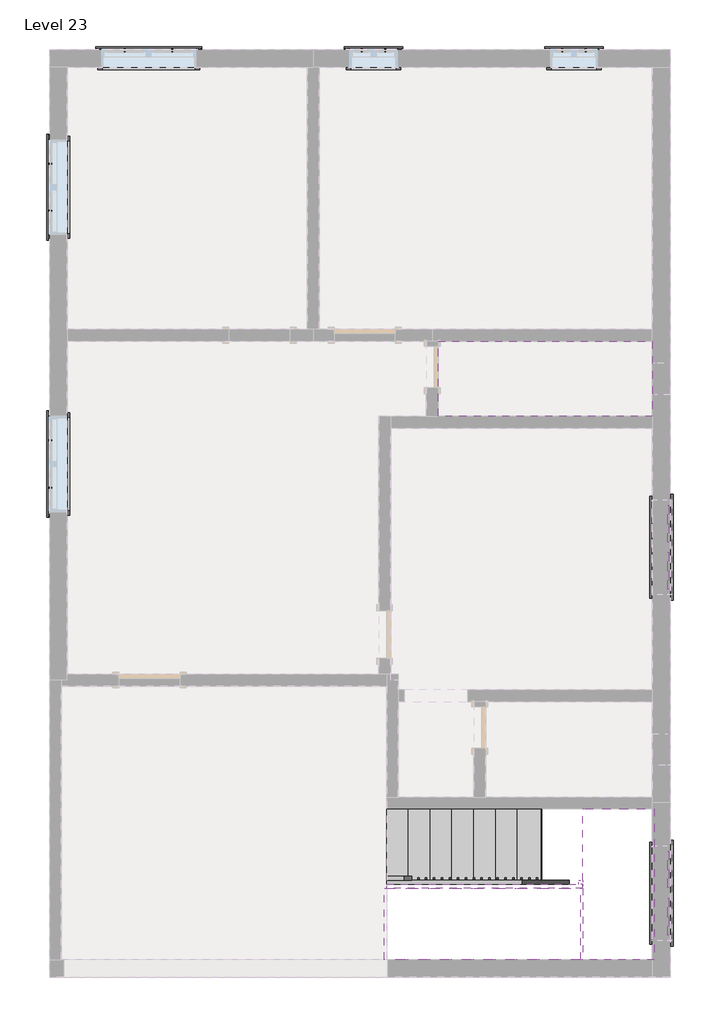
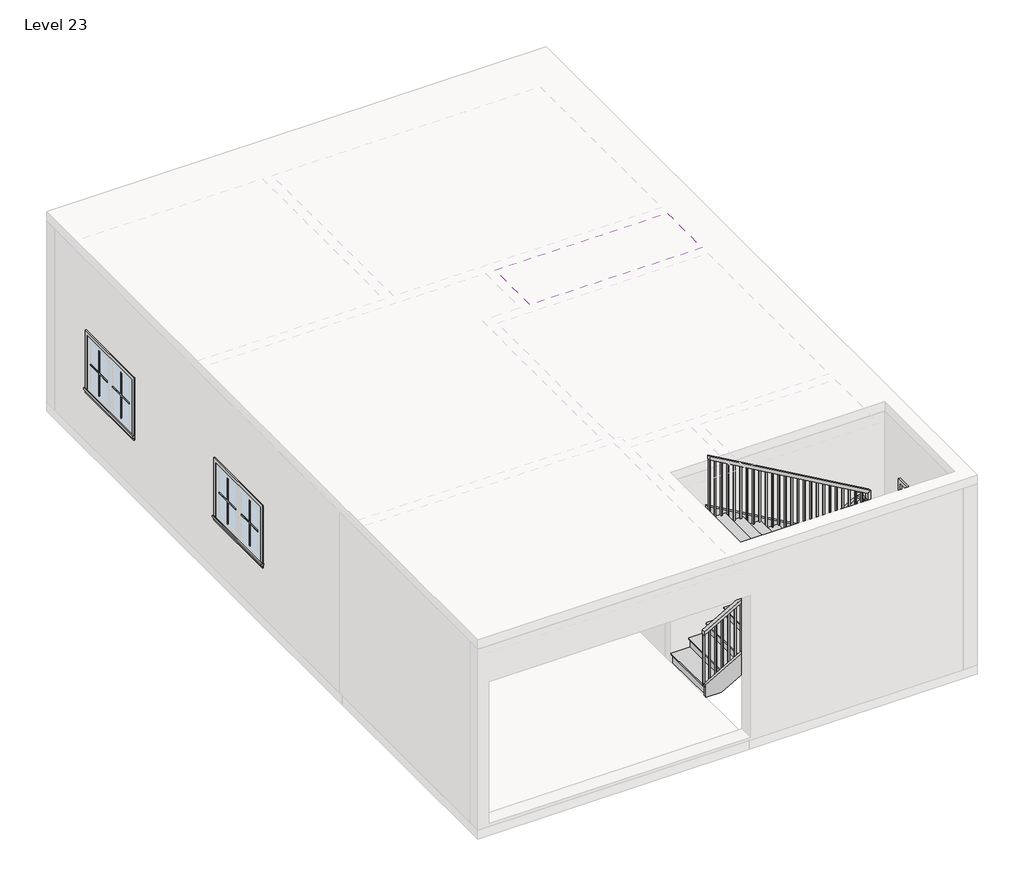
# One storey, part 2 of 2: 44 proxies, 3 members, 2 stair flights, 1 covering, 1 railing, 1 slab.
"""IFC4 building model written with IfcOpenShell, lengths in millimetres."""

from ifc_helpers import new_model, si_unit, frame, origin, place, context, project, spatial, polyline, outline, extrude, faceted_brep, transform, mapped, element, save
from components import muntin_pattern_2x2_muntin_pattern_2x2_2357e71d, muntin_pattern_2x2_muntin_pattern_2x2_302d8f29, muntin_pattern_2x2_muntin_pattern_2x2_53152e2c, muntin_pattern_2x2_muntin_pattern_2x2_e8f3e573, trim_window_exterior_flat_with_sill_c4e67c73, trim_window_exterior_flat_with_sill_a665a915, trim_window_interior_flat_picture_frame_cf1733af, trim_window_interior_flat_picture_frame_d485c387, non_monolithic_landing_f056e2ed, stair_flight_e0f3031c, stair_flight_f2ac7941

model = new_model("IFC4")

# Units and contexts
model_context = context("Model", 3, world=origin())
ifc_project = project(units=[si_unit("LENGTHUNIT", "METRE", prefix="MILLI")], contexts=[model_context])

# Site, building, storey
site = spatial("IfcSite", under=ifc_project)
building = spatial("IfcBuilding", under=site)
storey = spatial("IfcBuildingStorey", under=building, Name="Level 23", Elevation=19202.4)

# Proxies
placement = place(None, origin())
muntin_pattern_2x2_muntin_pattern_2x2_shape = muntin_pattern_2x2_muntin_pattern_2x2_2357e71d(model_context)
element("IfcBuildingElementProxy", 1, Name="Muntin Pattern_2x2 : Muntin Pattern_2x2", ObjectType="Muntin Pattern_2x2 : Muntin Pattern_2x2", at=placement, inside=storey, context=model_context, shape_type="MappedRepresentation", body=[
    mapped(muntin_pattern_2x2_muntin_pattern_2x2_shape, transform((-4942.3279463, 5897.3080275, 20186.65), x_axis=(1.0, 0.0, 0.0), y_axis=(0.0, 1.0, 0.0), z_axis=(0.0, 0.0, 1.0))),
])
element("IfcBuildingElementProxy", 2, Name="Muntin Pattern_2x2 : Muntin Pattern_2x2", ObjectType="Muntin Pattern_2x2 : Muntin Pattern_2x2", at=placement, inside=storey, context=model_context, shape_type="MappedRepresentation", body=[
    mapped(muntin_pattern_2x2_muntin_pattern_2x2_shape, transform((-5899.5904463, 3838.3205275, 20186.65), x_axis=(0.0, 1.0, 0.0), y_axis=(-1.0, 0.0, 0.0), z_axis=(0.0, 0.0, 1.0))),
])
element("IfcBuildingElementProxy", 3, Name="Muntin Pattern_2x2 : Muntin Pattern_2x2", ObjectType="Muntin Pattern_2x2 : Muntin Pattern_2x2", at=placement, inside=storey, context=model_context, shape_type="MappedRepresentation", body=[
    mapped(muntin_pattern_2x2_muntin_pattern_2x2_shape, transform((-5899.5904463, 293.4330275, 20186.65), x_axis=(0.0, 1.0, 0.0), y_axis=(-1.0, 0.0, 0.0), z_axis=(0.0, 0.0, 1.0))),
])
element("IfcBuildingElementProxy", 4, Name="Muntin Pattern_2x2 : Muntin Pattern_2x2", ObjectType="Muntin Pattern_2x2 : Muntin Pattern_2x2", at=placement, inside=storey, context=model_context, shape_type="MappedRepresentation", body=[
    mapped(muntin_pattern_2x2_muntin_pattern_2x2_shape, transform((2031.5595537, -166.9419725, 20491.45), x_axis=(0.0, -1.0, 0.0), y_axis=(1.0, 0.0, 0.0), z_axis=(0.0, 0.0, 1.0))),
])
element("IfcBuildingElementProxy", 5, Name="Muntin Pattern_2x2 : Muntin Pattern_2x2", ObjectType="Muntin Pattern_2x2 : Muntin Pattern_2x2", at=placement, inside=storey, context=model_context, shape_type="MappedRepresentation", body=[
    mapped(muntin_pattern_2x2_muntin_pattern_2x2_shape, transform((2031.5595537, -4599.2419725, 20491.45), x_axis=(0.0, -1.0, 0.0), y_axis=(1.0, 0.0, 0.0), z_axis=(0.0, 0.0, 1.0))),
])
element("IfcBuildingElementProxy", 6, Name="Muntin Pattern_2x2 : Muntin Pattern_2x2", ObjectType="Muntin Pattern_2x2 : Muntin Pattern_2x2", at=placement, inside=storey, context=model_context, shape_type="MappedRepresentation", body=[
    mapped(muntin_pattern_2x2_muntin_pattern_2x2_shape, transform((-4942.3279463, 5897.3080275, 20186.65), x_axis=(1.0, 0.0, 0.0), y_axis=(0.0, 1.0, 0.0), z_axis=(0.0, 0.0, 1.0))),
])
element("IfcBuildingElementProxy", 7, Name="Muntin Pattern_2x2 : Muntin Pattern_2x2", ObjectType="Muntin Pattern_2x2 : Muntin Pattern_2x2", at=placement, inside=storey, context=model_context, shape_type="MappedRepresentation", body=[
    mapped(muntin_pattern_2x2_muntin_pattern_2x2_shape, transform((2031.5595537, -4599.2419725, 20491.45), x_axis=(0.0, -1.0, 0.0), y_axis=(1.0, 0.0, 0.0), z_axis=(0.0, 0.0, 1.0))),
])
muntin_pattern_2x2_muntin_pattern_2x2_2_shape = muntin_pattern_2x2_muntin_pattern_2x2_302d8f29(model_context)
element("IfcBuildingElementProxy", 8, Name="Muntin Pattern_2x2 : Muntin Pattern_2x2", ObjectType="Muntin Pattern_2x2 : Muntin Pattern_2x2", at=placement, inside=storey, context=model_context, shape_type="MappedRepresentation", body=[
    mapped(muntin_pattern_2x2_muntin_pattern_2x2_2_shape, transform((-4335.9029463, 5897.3080275, 20186.65), x_axis=(-1.0, 0.0, 0.0), y_axis=(0.0, -1.0, 0.0), z_axis=(0.0, 0.0, 1.0))),
])
element("IfcBuildingElementProxy", 9, Name="Muntin Pattern_2x2 : Muntin Pattern_2x2", ObjectType="Muntin Pattern_2x2 : Muntin Pattern_2x2", at=placement, inside=storey, context=model_context, shape_type="MappedRepresentation", body=[
    mapped(muntin_pattern_2x2_muntin_pattern_2x2_2_shape, transform((-5899.5904463, 4444.7455275, 20186.65), x_axis=(0.0, -1.0, 0.0), y_axis=(1.0, 0.0, 0.0), z_axis=(0.0, 0.0, 1.0))),
])
element("IfcBuildingElementProxy", 10, Name="Muntin Pattern_2x2 : Muntin Pattern_2x2", ObjectType="Muntin Pattern_2x2 : Muntin Pattern_2x2", at=placement, inside=storey, context=model_context, shape_type="MappedRepresentation", body=[
    mapped(muntin_pattern_2x2_muntin_pattern_2x2_2_shape, transform((-5899.5904463, 899.8580275, 20186.65), x_axis=(0.0, -1.0, 0.0), y_axis=(1.0, 0.0, 0.0), z_axis=(0.0, 0.0, 1.0))),
])
element("IfcBuildingElementProxy", 11, Name="Muntin Pattern_2x2 : Muntin Pattern_2x2", ObjectType="Muntin Pattern_2x2 : Muntin Pattern_2x2", at=placement, inside=storey, context=model_context, shape_type="MappedRepresentation", body=[
    mapped(muntin_pattern_2x2_muntin_pattern_2x2_2_shape, transform((2031.5595537, -773.3669725, 20491.45), x_axis=(0.0, 1.0, 0.0), y_axis=(-1.0, 0.0, 0.0), z_axis=(0.0, 0.0, 1.0))),
])
element("IfcBuildingElementProxy", 12, Name="Muntin Pattern_2x2 : Muntin Pattern_2x2", ObjectType="Muntin Pattern_2x2 : Muntin Pattern_2x2", at=placement, inside=storey, context=model_context, shape_type="MappedRepresentation", body=[
    mapped(muntin_pattern_2x2_muntin_pattern_2x2_2_shape, transform((2031.5595537, -5205.6669725, 20491.45), x_axis=(0.0, 1.0, 0.0), y_axis=(-1.0, 0.0, 0.0), z_axis=(0.0, 0.0, 1.0))),
])
element("IfcBuildingElementProxy", 13, Name="Muntin Pattern_2x2 : Muntin Pattern_2x2", ObjectType="Muntin Pattern_2x2 : Muntin Pattern_2x2", at=placement, inside=storey, context=model_context, shape_type="MappedRepresentation", body=[
    mapped(muntin_pattern_2x2_muntin_pattern_2x2_2_shape, transform((-4335.9029463, 5897.3080275, 20186.65), x_axis=(-1.0, 0.0, 0.0), y_axis=(0.0, -1.0, 0.0), z_axis=(0.0, 0.0, 1.0))),
])
element("IfcBuildingElementProxy", 14, Name="Muntin Pattern_2x2 : Muntin Pattern_2x2", ObjectType="Muntin Pattern_2x2 : Muntin Pattern_2x2", at=placement, inside=storey, context=model_context, shape_type="MappedRepresentation", body=[
    mapped(muntin_pattern_2x2_muntin_pattern_2x2_2_shape, transform((2031.5595537, -5205.6669725, 20491.45), x_axis=(0.0, 1.0, 0.0), y_axis=(-1.0, 0.0, 0.0), z_axis=(0.0, 0.0, 1.0))),
])
muntin_pattern_2x2_muntin_pattern_2x2_3_shape = muntin_pattern_2x2_muntin_pattern_2x2_53152e2c(model_context)
element("IfcBuildingElementProxy", 15, Name="Muntin Pattern_2x2 : Muntin Pattern_2x2", ObjectType="Muntin Pattern_2x2 : Muntin Pattern_2x2", at=placement, inside=storey, context=model_context, shape_type="MappedRepresentation", body=[
    mapped(muntin_pattern_2x2_muntin_pattern_2x2_3_shape, transform((-1907.0279463, 5897.3080275, 20186.65), x_axis=(1.0, 0.0, 0.0), y_axis=(0.0, 1.0, 0.0), z_axis=(0.0, 0.0, 1.0))),
])
element("IfcBuildingElementProxy", 16, Name="Muntin Pattern_2x2 : Muntin Pattern_2x2", ObjectType="Muntin Pattern_2x2 : Muntin Pattern_2x2", at=placement, inside=storey, context=model_context, shape_type="MappedRepresentation", body=[
    mapped(muntin_pattern_2x2_muntin_pattern_2x2_3_shape, transform((658.3720537, 5897.3080275, 20186.65), x_axis=(1.0, 0.0, 0.0), y_axis=(0.0, 1.0, 0.0), z_axis=(0.0, 0.0, 1.0))),
])
element("IfcBuildingElementProxy", 17, Name="Muntin Pattern_2x2 : Muntin Pattern_2x2", ObjectType="Muntin Pattern_2x2 : Muntin Pattern_2x2", at=placement, inside=storey, context=model_context, shape_type="MappedRepresentation", body=[
    mapped(muntin_pattern_2x2_muntin_pattern_2x2_3_shape, transform((-1907.0279463, 5897.3080275, 20186.65), x_axis=(1.0, 0.0, 0.0), y_axis=(0.0, 1.0, 0.0), z_axis=(0.0, 0.0, 1.0))),
])
element("IfcBuildingElementProxy", 18, Name="Muntin Pattern_2x2 : Muntin Pattern_2x2", ObjectType="Muntin Pattern_2x2 : Muntin Pattern_2x2", at=placement, inside=storey, context=model_context, shape_type="MappedRepresentation", body=[
    mapped(muntin_pattern_2x2_muntin_pattern_2x2_3_shape, transform((658.3720537, 5897.3080275, 20186.65), x_axis=(1.0, 0.0, 0.0), y_axis=(0.0, 1.0, 0.0), z_axis=(0.0, 0.0, 1.0))),
])
muntin_pattern_2x2_muntin_pattern_2x2_4_shape = muntin_pattern_2x2_muntin_pattern_2x2_e8f3e573(model_context)
element("IfcBuildingElementProxy", 19, Name="Muntin Pattern_2x2 : Muntin Pattern_2x2", ObjectType="Muntin Pattern_2x2 : Muntin Pattern_2x2", at=placement, inside=storey, context=model_context, shape_type="MappedRepresentation", body=[
    mapped(muntin_pattern_2x2_muntin_pattern_2x2_4_shape, transform((-1605.4029463, 5897.3080275, 20186.65), x_axis=(-1.0, 0.0, 0.0), y_axis=(0.0, -1.0, 0.0), z_axis=(0.0, 0.0, 1.0))),
])
element("IfcBuildingElementProxy", 20, Name="Muntin Pattern_2x2 : Muntin Pattern_2x2", ObjectType="Muntin Pattern_2x2 : Muntin Pattern_2x2", at=placement, inside=storey, context=model_context, shape_type="MappedRepresentation", body=[
    mapped(muntin_pattern_2x2_muntin_pattern_2x2_4_shape, transform((959.9970537, 5897.3080275, 20186.65), x_axis=(-1.0, 0.0, 0.0), y_axis=(0.0, -1.0, 0.0), z_axis=(0.0, 0.0, 1.0))),
])
element("IfcBuildingElementProxy", 21, Name="Muntin Pattern_2x2 : Muntin Pattern_2x2", ObjectType="Muntin Pattern_2x2 : Muntin Pattern_2x2", at=placement, inside=storey, context=model_context, shape_type="MappedRepresentation", body=[
    mapped(muntin_pattern_2x2_muntin_pattern_2x2_4_shape, transform((-1605.4029463, 5897.3080275, 20186.65), x_axis=(-1.0, 0.0, 0.0), y_axis=(0.0, -1.0, 0.0), z_axis=(0.0, 0.0, 1.0))),
])
element("IfcBuildingElementProxy", 22, Name="Muntin Pattern_2x2 : Muntin Pattern_2x2", ObjectType="Muntin Pattern_2x2 : Muntin Pattern_2x2", at=placement, inside=storey, context=model_context, shape_type="MappedRepresentation", body=[
    mapped(muntin_pattern_2x2_muntin_pattern_2x2_4_shape, transform((959.9970537, 5897.3080275, 20186.65), x_axis=(-1.0, 0.0, 0.0), y_axis=(0.0, -1.0, 0.0), z_axis=(0.0, 0.0, 1.0))),
])
trim_window_exterior_flat_with_sill_shape = trim_window_exterior_flat_with_sill_c4e67c73(model_context)
element("IfcBuildingElementProxy", 23, Name="Trim-Window-Exterior-Flat : with Sill", ObjectType="Trim-Window-Exterior-Flat : with Sill", at=placement, inside=storey, context=model_context, shape_type="MappedRepresentation", body=[
    mapped(trim_window_exterior_flat_with_sill_shape, transform((-4639.1154463, 5906.8330275, 21031.2), x_axis=(-1.0, 0.0, 0.0), y_axis=(0.0, 0.0, 1.0), z_axis=(0.0, 1.0, 0.0))),
])
element("IfcBuildingElementProxy", 24, Name="Trim-Window-Exterior-Flat : with Sill", ObjectType="Trim-Window-Exterior-Flat : with Sill", at=placement, inside=storey, context=model_context, shape_type="MappedRepresentation", body=[
    mapped(trim_window_exterior_flat_with_sill_shape, transform((-5909.1154463, 4141.5330275, 21031.2), x_axis=(0.0, -1.0, 0.0), y_axis=(0.0, 0.0, 1.0), z_axis=(-1.0, 0.0, 0.0))),
])
element("IfcBuildingElementProxy", 25, Name="Trim-Window-Exterior-Flat : with Sill", ObjectType="Trim-Window-Exterior-Flat : with Sill", at=placement, inside=storey, context=model_context, shape_type="MappedRepresentation", body=[
    mapped(trim_window_exterior_flat_with_sill_shape, transform((-5909.1154463, 596.6455275, 21031.2), x_axis=(0.0, -1.0, 0.0), y_axis=(0.0, 0.0, 1.0), z_axis=(-1.0, 0.0, 0.0))),
])
element("IfcBuildingElementProxy", 26, Name="Trim-Window-Exterior-Flat : with Sill", ObjectType="Trim-Window-Exterior-Flat : with Sill", at=placement, inside=storey, context=model_context, shape_type="MappedRepresentation", body=[
    mapped(trim_window_exterior_flat_with_sill_shape, transform((2041.0845537, -470.1544725, 21336.0), x_axis=(0.0, 1.0, 0.0), y_axis=(0.0, 0.0, 1.0), z_axis=(1.0, 0.0, 0.0))),
])
element("IfcBuildingElementProxy", 27, Name="Trim-Window-Exterior-Flat : with Sill", ObjectType="Trim-Window-Exterior-Flat : with Sill", at=placement, inside=storey, context=model_context, shape_type="MappedRepresentation", body=[
    mapped(trim_window_exterior_flat_with_sill_shape, transform((2041.0845537, -4902.4544725, 21336.0), x_axis=(0.0, 1.0, 0.0), y_axis=(0.0, 0.0, 1.0), z_axis=(1.0, 0.0, 0.0))),
])
element("IfcBuildingElementProxy", 28, Name="Trim-Window-Exterior-Flat : with Sill", ObjectType="Trim-Window-Exterior-Flat : with Sill", at=placement, inside=storey, context=model_context, shape_type="MappedRepresentation", body=[
    mapped(trim_window_exterior_flat_with_sill_shape, transform((-4639.1154463, 5906.8330275, 21031.2), x_axis=(-1.0, 0.0, 0.0), y_axis=(0.0, 0.0, 1.0), z_axis=(0.0, 1.0, 0.0))),
])
element("IfcBuildingElementProxy", 29, Name="Trim-Window-Exterior-Flat : with Sill", ObjectType="Trim-Window-Exterior-Flat : with Sill", at=placement, inside=storey, context=model_context, shape_type="MappedRepresentation", body=[
    mapped(trim_window_exterior_flat_with_sill_shape, transform((2041.0845537, -4902.4544725, 21336.0), x_axis=(0.0, 1.0, 0.0), y_axis=(0.0, 0.0, 1.0), z_axis=(1.0, 0.0, 0.0))),
])
trim_window_exterior_flat_with_sill_2_shape = trim_window_exterior_flat_with_sill_a665a915(model_context)
element("IfcBuildingElementProxy", 30, Name="Trim-Window-Exterior-Flat : with Sill", ObjectType="Trim-Window-Exterior-Flat : with Sill", at=placement, inside=storey, context=model_context, shape_type="MappedRepresentation", body=[
    mapped(trim_window_exterior_flat_with_sill_2_shape, transform((-1756.2154463, 5906.8330275, 21031.2), x_axis=(-1.0, 0.0, 0.0), y_axis=(0.0, 0.0, 1.0), z_axis=(0.0, 1.0, 0.0))),
])
element("IfcBuildingElementProxy", 31, Name="Trim-Window-Exterior-Flat : with Sill", ObjectType="Trim-Window-Exterior-Flat : with Sill", at=placement, inside=storey, context=model_context, shape_type="MappedRepresentation", body=[
    mapped(trim_window_exterior_flat_with_sill_2_shape, transform((809.1845537, 5906.8330275, 21031.2), x_axis=(-1.0, 0.0, 0.0), y_axis=(0.0, 0.0, 1.0), z_axis=(0.0, 1.0, 0.0))),
])
element("IfcBuildingElementProxy", 32, Name="Trim-Window-Exterior-Flat : with Sill", ObjectType="Trim-Window-Exterior-Flat : with Sill", at=placement, inside=storey, context=model_context, shape_type="MappedRepresentation", body=[
    mapped(trim_window_exterior_flat_with_sill_2_shape, transform((-1756.2154463, 5906.8330275, 21031.2), x_axis=(-1.0, 0.0, 0.0), y_axis=(0.0, 0.0, 1.0), z_axis=(0.0, 1.0, 0.0))),
])
element("IfcBuildingElementProxy", 33, Name="Trim-Window-Exterior-Flat : with Sill", ObjectType="Trim-Window-Exterior-Flat : with Sill", at=placement, inside=storey, context=model_context, shape_type="MappedRepresentation", body=[
    mapped(trim_window_exterior_flat_with_sill_2_shape, transform((809.1845537, 5906.8330275, 21031.2), x_axis=(-1.0, 0.0, 0.0), y_axis=(0.0, 0.0, 1.0), z_axis=(0.0, 1.0, 0.0))),
])
trim_window_interior_flat_picture_frame_shape = trim_window_interior_flat_picture_frame_cf1733af(model_context)
element("IfcBuildingElementProxy", 34, Name="Trim-Window-Interior-Flat : Picture Frame", ObjectType="Trim-Window-Interior-Flat : Picture Frame", at=placement, inside=storey, context=model_context, shape_type="MappedRepresentation", body=[
    mapped(trim_window_interior_flat_picture_frame_shape, transform((-4639.1154463, 5678.2330275, 21031.2), x_axis=(1.0, 0.0, 0.0), y_axis=(0.0, 0.0, 1.0), z_axis=(0.0, -1.0, 0.0))),
])
element("IfcBuildingElementProxy", 35, Name="Trim-Window-Interior-Flat : Picture Frame", ObjectType="Trim-Window-Interior-Flat : Picture Frame", at=placement, inside=storey, context=model_context, shape_type="MappedRepresentation", body=[
    mapped(trim_window_interior_flat_picture_frame_shape, transform((-5680.5154463, 4141.5330275, 21031.2), x_axis=(0.0, 1.0, 0.0), y_axis=(0.0, 0.0, 1.0), z_axis=(1.0, 0.0, 0.0))),
])
element("IfcBuildingElementProxy", 36, Name="Trim-Window-Interior-Flat : Picture Frame", ObjectType="Trim-Window-Interior-Flat : Picture Frame", at=placement, inside=storey, context=model_context, shape_type="MappedRepresentation", body=[
    mapped(trim_window_interior_flat_picture_frame_shape, transform((-5680.5154463, 596.6455275, 21031.2), x_axis=(0.0, 1.0, 0.0), y_axis=(0.0, 0.0, 1.0), z_axis=(1.0, 0.0, 0.0))),
])
element("IfcBuildingElementProxy", 37, Name="Trim-Window-Interior-Flat : Picture Frame", ObjectType="Trim-Window-Interior-Flat : Picture Frame", at=placement, inside=storey, context=model_context, shape_type="MappedRepresentation", body=[
    mapped(trim_window_interior_flat_picture_frame_shape, transform((1812.4845537, -470.1544725, 21336.0), x_axis=(0.0, -1.0, 0.0), y_axis=(0.0, 0.0, 1.0), z_axis=(-1.0, 0.0, 0.0))),
])
element("IfcBuildingElementProxy", 38, Name="Trim-Window-Interior-Flat : Picture Frame", ObjectType="Trim-Window-Interior-Flat : Picture Frame", at=placement, inside=storey, context=model_context, shape_type="MappedRepresentation", body=[
    mapped(trim_window_interior_flat_picture_frame_shape, transform((1812.4845537, -4902.4544725, 21336.0), x_axis=(0.0, -1.0, 0.0), y_axis=(0.0, 0.0, 1.0), z_axis=(-1.0, 0.0, 0.0))),
])
element("IfcBuildingElementProxy", 39, Name="Trim-Window-Interior-Flat : Picture Frame", ObjectType="Trim-Window-Interior-Flat : Picture Frame", at=placement, inside=storey, context=model_context, shape_type="MappedRepresentation", body=[
    mapped(trim_window_interior_flat_picture_frame_shape, transform((-4639.1154463, 5678.2330275, 21031.2), x_axis=(1.0, 0.0, 0.0), y_axis=(0.0, 0.0, 1.0), z_axis=(0.0, -1.0, 0.0))),
])
element("IfcBuildingElementProxy", 40, Name="Trim-Window-Interior-Flat : Picture Frame", ObjectType="Trim-Window-Interior-Flat : Picture Frame", at=placement, inside=storey, context=model_context, shape_type="MappedRepresentation", body=[
    mapped(trim_window_interior_flat_picture_frame_shape, transform((1812.4845537, -4902.4544725, 21336.0), x_axis=(0.0, -1.0, 0.0), y_axis=(0.0, 0.0, 1.0), z_axis=(-1.0, 0.0, 0.0))),
])
trim_window_interior_flat_picture_frame_2_shape = trim_window_interior_flat_picture_frame_d485c387(model_context)
element("IfcBuildingElementProxy", 41, Name="Trim-Window-Interior-Flat : Picture Frame", ObjectType="Trim-Window-Interior-Flat : Picture Frame", at=placement, inside=storey, context=model_context, shape_type="MappedRepresentation", body=[
    mapped(trim_window_interior_flat_picture_frame_2_shape, transform((-1756.2154463, 5678.2330275, 21031.2), x_axis=(1.0, 0.0, 0.0), y_axis=(0.0, 0.0, 1.0), z_axis=(0.0, -1.0, 0.0))),
])
element("IfcBuildingElementProxy", 42, Name="Trim-Window-Interior-Flat : Picture Frame", ObjectType="Trim-Window-Interior-Flat : Picture Frame", at=placement, inside=storey, context=model_context, shape_type="MappedRepresentation", body=[
    mapped(trim_window_interior_flat_picture_frame_2_shape, transform((809.1845537, 5678.2330275, 21031.2), x_axis=(1.0, 0.0, 0.0), y_axis=(0.0, 0.0, 1.0), z_axis=(0.0, -1.0, 0.0))),
])
element("IfcBuildingElementProxy", 43, Name="Trim-Window-Interior-Flat : Picture Frame", ObjectType="Trim-Window-Interior-Flat : Picture Frame", at=placement, inside=storey, context=model_context, shape_type="MappedRepresentation", body=[
    mapped(trim_window_interior_flat_picture_frame_2_shape, transform((-1756.2154463, 5678.2330275, 21031.2), x_axis=(1.0, 0.0, 0.0), y_axis=(0.0, 0.0, 1.0), z_axis=(0.0, -1.0, 0.0))),
])
element("IfcBuildingElementProxy", 44, Name="Trim-Window-Interior-Flat : Picture Frame", ObjectType="Trim-Window-Interior-Flat : Picture Frame", at=placement, inside=storey, context=model_context, shape_type="MappedRepresentation", body=[
    mapped(trim_window_interior_flat_picture_frame_2_shape, transform((809.1845537, 5678.2330275, 21031.2), x_axis=(1.0, 0.0, 0.0), y_axis=(0.0, 0.0, 1.0), z_axis=(0.0, -1.0, 0.0))),
])

# Covering
element("IfcCovering", 45, ObjectType="2' x 4' ACT System", at=placement, inside=storey, context=model_context, shape_type="SweptSolid", body=[
    extrude(outline(polyline([(-930.7154463, 2171.4455275), (1812.4845537, 2171.4455275), (1812.4845537, 1206.2455275), (-930.7154463, 1206.2455275), (-930.7154463, 2171.4455275)])), frame((0.0, 0.0, 21945.6), z_axis=(0.0, 0.0, 1.0), x_axis=(1.0, 0.0, 0.0)), (0.0, 0.0, 1.0), 57.15),
])

# Members
element("IfcMember", 46, ObjectType="Stringer - 2\" Width", at=placement, inside=storey, context=model_context, shape_type="SweptSolid", body=[
    extrude(outline(polyline([(19411.4890626, -1591.1154463), (19202.4, -1591.1154463), (19202.4, -1342.8974141), (20471.324218, 872.6845537), (20822.5745172, 872.6845537), (19411.4890626, -1591.1154463)])), frame((0.0, -4788.1544725, 0.0), z_axis=(0.0, 1.0, 0.0), x_axis=(0.0, 0.0, 1.0)), (0.0, 0.0, 1.0), 50.8),
])
element("IfcMember", 47, ObjectType="Stringer - 2\" Width", at=placement, inside=storey, context=model_context, shape_type="SweptSolid", body=[
    extrude(outline(polyline([(20660.4387634, 923.4845537), (21011.6890626, 923.4845537), (22451.8690626, -1591.1154463), (22100.6187634, -1591.1154463), (20660.4387634, 923.4845537)])), frame((0.0, -4838.9544725, 0.0), z_axis=(0.0, 1.0, 0.0), x_axis=(0.0, 0.0, 1.0)), (0.0, 0.0, 1.0), 50.8),
])
element("IfcMember", 48, ObjectType="Stringer - 2\" Width", at=placement, inside=storey, context=model_context, shape_type="SweptSolid", body=[
    extrude(outline(polyline([(872.6845537, -4737.3544725), (923.4845537, -4737.3544725), (923.4845537, -4788.1544725), (872.6845537, -4788.1544725), (872.6845537, -4737.3544725)])), frame((0.0, 0.0, 20574.0), z_axis=(0.0, 0.0, 1.0), x_axis=(1.0, 0.0, 0.0)), (0.0, 0.0, 1.0), 304.8),
])

# Railing
element("IfcRailing", 49, ObjectType="Handrail - Rectangular", at=placement, inside=storey, context=model_context, shape_type="SolidModel", body=[
    faceted_brep([(-1591.1154463, -4686.5544725, 20276.82), (-1591.1154463, -4686.5544725, 20218.2782835), (-1591.1154463, -4737.3544725, 20218.2782835), (-1591.1154463, -4737.3544725, 20276.82), (847.2845537, -4686.5544725, 21673.3581818), (898.0845537, -4686.5544725, 21643.9110107), (898.0845537, -4737.3544725, 21643.9110107), (847.2845537, -4737.3544725, 21673.3581818), (847.2845537, -4686.5544725, 21717.0), (898.0845537, -4686.5544725, 21666.2), (898.0845537, -4737.3544725, 21666.2), (847.2845537, -4737.3544725, 21717.0), (974.2845537, -4686.5544725, 21717.0), (974.2845537, -4686.5544725, 21666.2), (923.4845537, -4737.3544725, 21666.2), (923.4845537, -4737.3544725, 21717.0), (974.2845537, -4813.5544725, 21717.0), (974.2845537, -4813.5544725, 21666.2), (923.4845537, -4813.5544725, 21666.2), (923.4845537, -4813.5544725, 21717.0), (974.2845537, -4838.9544725, 21717.0), (923.4845537, -4838.9544725, 21717.0), (923.4845537, -4889.7544725, 21666.2), (974.2845537, -4889.7544725, 21666.2)], [[[0, 1, 2, 3]], [[1, 0, 4, 5]], [[2, 1, 5, 6]], [[3, 2, 6, 7]], [[0, 3, 7, 4]], [[5, 4, 8, 9]], [[6, 5, 9, 10]], [[7, 6, 10, 11]], [[4, 7, 11, 8]], [[9, 8, 12, 13]], [[10, 9, 13, 14]], [[11, 10, 14, 15]], [[8, 11, 15, 12]], [[13, 12, 16, 17]], [[14, 13, 17, 18]], [[15, 14, 18, 19]], [[12, 15, 19, 16]], [[20, 21, 22, 23]], [[17, 16, 20, 23]], [[18, 17, 23, 22]], [[19, 18, 22, 21]], [[16, 19, 21, 20]]]),
    faceted_brep([(974.2845537, -4838.9544725, 21717.0), (974.2845537, -4889.7544725, 21666.2), (923.4845537, -4889.7544725, 21666.2), (923.4845537, -4838.9544725, 21717.0), (974.2845537, -4838.9544725, 21847.9254545), (923.4845537, -4838.9544725, 21818.4782835), (923.4845537, -4889.7544725, 21818.4782835), (974.2845537, -4889.7544725, 21847.9254545)], [[[0, 1, 2, 3]], [[4, 5, 6, 7]], [[1, 0, 4, 7]], [[2, 1, 7, 6]], [[3, 2, 6, 5]], [[0, 3, 5, 4]]]),
    faceted_brep([(974.2845537, -4889.7544725, 21847.9254545), (923.4845537, -4889.7544725, 21818.4782835), (923.4845537, -4838.9544725, 21818.4782835), (974.2845537, -4838.9544725, 21847.9254545), (-1591.1154463, -4889.7544725, 23317.2), (-1591.1154463, -4838.9544725, 23317.2), (-1591.1154463, -4838.9544725, 23258.6582835), (-1591.1154463, -4889.7544725, 23258.6582835)], [[[0, 1, 2, 3]], [[4, 5, 6, 7]], [[1, 0, 4, 7]], [[2, 1, 7, 6]], [[3, 2, 6, 5]], [[0, 3, 5, 4]]]),
    extrude(outline(polyline([(23195.0139653, -1479.9904463), (23205.9244198, -1499.0404463), (22242.78, -1499.0404463), (22242.78, -1479.9904463), (23195.0139653, -1479.9904463)])), frame((0.0, -4873.8794725, 0.0), z_axis=(0.0, 1.0, 0.0), x_axis=(0.0, 0.0, 1.0)), (0.0, 0.0, 1.0), 19.05),
    extrude(outline(polyline([(23136.8248744, -1378.3904463), (23147.7353289, -1397.4404463), (22242.78, -1397.4404463), (22242.78, -1378.3904463), (23136.8248744, -1378.3904463)])), frame((0.0, -4873.8794725, 0.0), z_axis=(0.0, 1.0, 0.0), x_axis=(0.0, 0.0, 1.0)), (0.0, 0.0, 1.0), 19.05),
    extrude(outline(polyline([(23078.6357835, -1276.7904463), (23089.546238, -1295.8404463), (22082.76, -1295.8404463), (22082.76, -1276.7904463), (23078.6357835, -1276.7904463)])), frame((0.0, -4873.8794725, 0.0), z_axis=(0.0, 1.0, 0.0), x_axis=(0.0, 0.0, 1.0)), (0.0, 0.0, 1.0), 19.05),
    extrude(outline(polyline([(23020.4466926, -1175.1904463), (23031.3571471, -1194.2404463), (22082.76, -1194.2404463), (22082.76, -1175.1904463), (23020.4466926, -1175.1904463)])), frame((0.0, -4873.8794725, 0.0), z_axis=(0.0, 1.0, 0.0), x_axis=(0.0, 0.0, 1.0)), (0.0, 0.0, 1.0), 19.05),
    extrude(outline(polyline([(22962.2576016, -1073.5904463), (22973.1680562, -1092.6404463), (22082.76, -1092.6404463), (22082.76, -1073.5904463), (22962.2576016, -1073.5904463)])), frame((0.0, -4873.8794725, 0.0), z_axis=(0.0, 1.0, 0.0), x_axis=(0.0, 0.0, 1.0)), (0.0, 0.0, 1.0), 19.05),
    extrude(outline(polyline([(22904.0685107, -971.9904463), (22914.9789653, -991.0404463), (21922.74, -991.0404463), (21922.74, -971.9904463), (22904.0685107, -971.9904463)])), frame((0.0, -4873.8794725, 0.0), z_axis=(0.0, 1.0, 0.0), x_axis=(0.0, 0.0, 1.0)), (0.0, 0.0, 1.0), 19.05),
    extrude(outline(polyline([(22845.8794198, -870.3904463), (22856.7898744, -889.4404463), (21922.74, -889.4404463), (21922.74, -870.3904463), (22845.8794198, -870.3904463)])), frame((0.0, -4873.8794725, 0.0), z_axis=(0.0, 1.0, 0.0), x_axis=(0.0, 0.0, 1.0)), (0.0, 0.0, 1.0), 19.05),
    extrude(outline(polyline([(22787.6903289, -768.7904463), (22798.6007835, -787.8404463), (21922.74, -787.8404463), (21922.74, -768.7904463), (22787.6903289, -768.7904463)])), frame((0.0, -4873.8794725, 0.0), z_axis=(0.0, 1.0, 0.0), x_axis=(0.0, 0.0, 1.0)), (0.0, 0.0, 1.0), 19.05),
    extrude(outline(polyline([(22729.501238, -667.1904463), (22740.4116926, -686.2404463), (21762.72, -686.2404463), (21762.72, -667.1904463), (22729.501238, -667.1904463)])), frame((0.0, -4873.8794725, 0.0), z_axis=(0.0, 1.0, 0.0), x_axis=(0.0, 0.0, 1.0)), (0.0, 0.0, 1.0), 19.05),
    extrude(outline(polyline([(22671.3121471, -565.5904463), (22682.2226016, -584.6404463), (21762.72, -584.6404463), (21762.72, -565.5904463), (22671.3121471, -565.5904463)])), frame((0.0, -4873.8794725, 0.0), z_axis=(0.0, 1.0, 0.0), x_axis=(0.0, 0.0, 1.0)), (0.0, 0.0, 1.0), 19.05),
    extrude(outline(polyline([(22613.1230562, -463.9904463), (22624.0335107, -483.0404463), (21762.72, -483.0404463), (21762.72, -463.9904463), (22613.1230562, -463.9904463)])), frame((0.0, -4873.8794725, 0.0), z_axis=(0.0, 1.0, 0.0), x_axis=(0.0, 0.0, 1.0)), (0.0, 0.0, 1.0), 19.05),
    extrude(outline(polyline([(22554.9339653, -362.3904463), (22565.8444198, -381.4404463), (21602.7, -381.4404463), (21602.7, -362.3904463), (22554.9339653, -362.3904463)])), frame((0.0, -4873.8794725, 0.0), z_axis=(0.0, 1.0, 0.0), x_axis=(0.0, 0.0, 1.0)), (0.0, 0.0, 1.0), 19.05),
    extrude(outline(polyline([(22496.7448744, -260.7904463), (22507.6553289, -279.8404463), (21602.7, -279.8404463), (21602.7, -260.7904463), (22496.7448744, -260.7904463)])), frame((0.0, -4873.8794725, 0.0), z_axis=(0.0, 1.0, 0.0), x_axis=(0.0, 0.0, 1.0)), (0.0, 0.0, 1.0), 19.05),
    extrude(outline(polyline([(22438.5557835, -159.1904463), (22449.466238, -178.2404463), (21442.68, -178.2404463), (21442.68, -159.1904463), (22438.5557835, -159.1904463)])), frame((0.0, -4873.8794725, 0.0), z_axis=(0.0, 1.0, 0.0), x_axis=(0.0, 0.0, 1.0)), (0.0, 0.0, 1.0), 19.05),
    extrude(outline(polyline([(22380.3666926, -57.5904463), (22391.2771471, -76.6404463), (21442.68, -76.6404463), (21442.68, -57.5904463), (22380.3666926, -57.5904463)])), frame((0.0, -4873.8794725, 0.0), z_axis=(0.0, 1.0, 0.0), x_axis=(0.0, 0.0, 1.0)), (0.0, 0.0, 1.0), 19.05),
    extrude(outline(polyline([(22322.1776016, 44.0095537), (22333.0880562, 24.9595537), (21442.68, 24.9595537), (21442.68, 44.0095537), (22322.1776016, 44.0095537)])), frame((0.0, -4873.8794725, 0.0), z_axis=(0.0, 1.0, 0.0), x_axis=(0.0, 0.0, 1.0)), (0.0, 0.0, 1.0), 19.05),
    extrude(outline(polyline([(22263.9885107, 145.6095537), (22274.8989653, 126.5595537), (21282.66, 126.5595537), (21282.66, 145.6095537), (22263.9885107, 145.6095537)])), frame((0.0, -4873.8794725, 0.0), z_axis=(0.0, 1.0, 0.0), x_axis=(0.0, 0.0, 1.0)), (0.0, 0.0, 1.0), 19.05),
    extrude(outline(polyline([(22205.7994198, 247.2095537), (22216.7098744, 228.1595537), (21282.66, 228.1595537), (21282.66, 247.2095537), (22205.7994198, 247.2095537)])), frame((0.0, -4873.8794725, 0.0), z_axis=(0.0, 1.0, 0.0), x_axis=(0.0, 0.0, 1.0)), (0.0, 0.0, 1.0), 19.05),
    extrude(outline(polyline([(22147.6103289, 348.8095537), (22158.5207835, 329.7595537), (21282.66, 329.7595537), (21282.66, 348.8095537), (22147.6103289, 348.8095537)])), frame((0.0, -4873.8794725, 0.0), z_axis=(0.0, 1.0, 0.0), x_axis=(0.0, 0.0, 1.0)), (0.0, 0.0, 1.0), 19.05),
    extrude(outline(polyline([(22089.421238, 450.4095537), (22100.3316926, 431.3595537), (21122.64, 431.3595537), (21122.64, 450.4095537), (22089.421238, 450.4095537)])), frame((0.0, -4873.8794725, 0.0), z_axis=(0.0, 1.0, 0.0), x_axis=(0.0, 0.0, 1.0)), (0.0, 0.0, 1.0), 19.05),
    extrude(outline(polyline([(22031.2321471, 552.0095537), (22042.1426016, 532.9595537), (21122.64, 532.9595537), (21122.64, 552.0095537), (22031.2321471, 552.0095537)])), frame((0.0, -4873.8794725, 0.0), z_axis=(0.0, 1.0, 0.0), x_axis=(0.0, 0.0, 1.0)), (0.0, 0.0, 1.0), 19.05),
    extrude(outline(polyline([(21973.0430562, 653.6095537), (21983.9535107, 634.5595537), (21122.64, 634.5595537), (21122.64, 653.6095537), (21973.0430562, 653.6095537)])), frame((0.0, -4873.8794725, 0.0), z_axis=(0.0, 1.0, 0.0), x_axis=(0.0, 0.0, 1.0)), (0.0, 0.0, 1.0), 19.05),
    extrude(outline(polyline([(21914.8539653, 755.2095537), (21925.7644198, 736.1595537), (20962.62, 736.1595537), (20962.62, 755.2095537), (21914.8539653, 755.2095537)])), frame((0.0, -4873.8794725, 0.0), z_axis=(0.0, 1.0, 0.0), x_axis=(0.0, 0.0, 1.0)), (0.0, 0.0, 1.0), 19.05),
    extrude(outline(polyline([(21856.6648744, 856.8095537), (21867.5753289, 837.7595537), (20962.62, 837.7595537), (20962.62, 856.8095537), (21856.6648744, 856.8095537)])), frame((0.0, -4873.8794725, 0.0), z_axis=(0.0, 1.0, 0.0), x_axis=(0.0, 0.0, 1.0)), (0.0, 0.0, 1.0), 19.05),
    extrude(outline(polyline([(939.3595537, -4804.0294725), (958.4095537, -4804.0294725), (958.4095537, -4823.0794725), (939.3595537, -4823.0794725), (939.3595537, -4804.0294725)])), frame((0.0, 0.0, 20802.6), z_axis=(0.0, 0.0, 1.0), x_axis=(1.0, 0.0, 0.0)), (0.0, 0.0, 1.0), 863.6),
    extrude(outline(polyline([(21620.2716926, 856.8095537), (21609.361238, 837.7595537), (20642.58, 837.7595537), (20642.58, 856.8095537), (21620.2716926, 856.8095537)])), frame((0.0, -4721.4794725, 0.0), z_axis=(0.0, 1.0, 0.0), x_axis=(0.0, 0.0, 1.0)), (0.0, 0.0, 1.0), 19.05),
    extrude(outline(polyline([(21562.0826016, 755.2095537), (21551.1721471, 736.1595537), (20642.58, 736.1595537), (20642.58, 755.2095537), (21562.0826016, 755.2095537)])), frame((0.0, -4721.4794725, 0.0), z_axis=(0.0, 1.0, 0.0), x_axis=(0.0, 0.0, 1.0)), (0.0, 0.0, 1.0), 19.05),
    extrude(outline(polyline([(21503.8935107, 653.6095537), (21492.9830562, 634.5595537), (20642.58, 634.5595537), (20642.58, 653.6095537), (21503.8935107, 653.6095537)])), frame((0.0, -4721.4794725, 0.0), z_axis=(0.0, 1.0, 0.0), x_axis=(0.0, 0.0, 1.0)), (0.0, 0.0, 1.0), 19.05),
    extrude(outline(polyline([(21445.7044198, 552.0095537), (21434.7939653, 532.9595537), (20482.56, 532.9595537), (20482.56, 552.0095537), (21445.7044198, 552.0095537)])), frame((0.0, -4721.4794725, 0.0), z_axis=(0.0, 1.0, 0.0), x_axis=(0.0, 0.0, 1.0)), (0.0, 0.0, 1.0), 19.05),
    extrude(outline(polyline([(21387.5153289, 450.4095537), (21376.6048744, 431.3595537), (20482.56, 431.3595537), (20482.56, 450.4095537), (21387.5153289, 450.4095537)])), frame((0.0, -4721.4794725, 0.0), z_axis=(0.0, 1.0, 0.0), x_axis=(0.0, 0.0, 1.0)), (0.0, 0.0, 1.0), 19.05),
    extrude(outline(polyline([(21329.326238, 348.8095537), (21318.4157835, 329.7595537), (20322.54, 329.7595537), (20322.54, 348.8095537), (21329.326238, 348.8095537)])), frame((0.0, -4721.4794725, 0.0), z_axis=(0.0, 1.0, 0.0), x_axis=(0.0, 0.0, 1.0)), (0.0, 0.0, 1.0), 19.05),
    extrude(outline(polyline([(21271.1371471, 247.2095537), (21260.2266926, 228.1595537), (20322.54, 228.1595537), (20322.54, 247.2095537), (21271.1371471, 247.2095537)])), frame((0.0, -4721.4794725, 0.0), z_axis=(0.0, 1.0, 0.0), x_axis=(0.0, 0.0, 1.0)), (0.0, 0.0, 1.0), 19.05),
    extrude(outline(polyline([(21212.9480562, 145.6095537), (21202.0376016, 126.5595537), (20322.54, 126.5595537), (20322.54, 145.6095537), (21212.9480562, 145.6095537)])), frame((0.0, -4721.4794725, 0.0), z_axis=(0.0, 1.0, 0.0), x_axis=(0.0, 0.0, 1.0)), (0.0, 0.0, 1.0), 19.05),
    extrude(outline(polyline([(21154.7589653, 44.0095537), (21143.8485107, 24.9595537), (20162.52, 24.9595537), (20162.52, 44.0095537), (21154.7589653, 44.0095537)])), frame((0.0, -4721.4794725, 0.0), z_axis=(0.0, 1.0, 0.0), x_axis=(0.0, 0.0, 1.0)), (0.0, 0.0, 1.0), 19.05),
    extrude(outline(polyline([(21096.5698744, -57.5904463), (21085.6594198, -76.6404463), (20162.52, -76.6404463), (20162.52, -57.5904463), (21096.5698744, -57.5904463)])), frame((0.0, -4721.4794725, 0.0), z_axis=(0.0, 1.0, 0.0), x_axis=(0.0, 0.0, 1.0)), (0.0, 0.0, 1.0), 19.05),
    extrude(outline(polyline([(21038.3807835, -159.1904463), (21027.4703289, -178.2404463), (20162.52, -178.2404463), (20162.52, -159.1904463), (21038.3807835, -159.1904463)])), frame((0.0, -4721.4794725, 0.0), z_axis=(0.0, 1.0, 0.0), x_axis=(0.0, 0.0, 1.0)), (0.0, 0.0, 1.0), 19.05),
    extrude(outline(polyline([(20980.1916926, -260.7904463), (20969.281238, -279.8404463), (20002.5, -279.8404463), (20002.5, -260.7904463), (20980.1916926, -260.7904463)])), frame((0.0, -4721.4794725, 0.0), z_axis=(0.0, 1.0, 0.0), x_axis=(0.0, 0.0, 1.0)), (0.0, 0.0, 1.0), 19.05),
    extrude(outline(polyline([(20922.0026016, -362.3904463), (20911.0921471, -381.4404463), (20002.5, -381.4404463), (20002.5, -362.3904463), (20922.0026016, -362.3904463)])), frame((0.0, -4721.4794725, 0.0), z_axis=(0.0, 1.0, 0.0), x_axis=(0.0, 0.0, 1.0)), (0.0, 0.0, 1.0), 19.05),
    extrude(outline(polyline([(20863.8135107, -463.9904463), (20852.9030562, -483.0404463), (20002.5, -483.0404463), (20002.5, -463.9904463), (20863.8135107, -463.9904463)])), frame((0.0, -4721.4794725, 0.0), z_axis=(0.0, 1.0, 0.0), x_axis=(0.0, 0.0, 1.0)), (0.0, 0.0, 1.0), 19.05),
    extrude(outline(polyline([(20805.6244198, -565.5904463), (20794.7139653, -584.6404463), (19842.48, -584.6404463), (19842.48, -565.5904463), (20805.6244198, -565.5904463)])), frame((0.0, -4721.4794725, 0.0), z_axis=(0.0, 1.0, 0.0), x_axis=(0.0, 0.0, 1.0)), (0.0, 0.0, 1.0), 19.05),
    extrude(outline(polyline([(20747.4353289, -667.1904463), (20736.5248744, -686.2404463), (19842.48, -686.2404463), (19842.48, -667.1904463), (20747.4353289, -667.1904463)])), frame((0.0, -4721.4794725, 0.0), z_axis=(0.0, 1.0, 0.0), x_axis=(0.0, 0.0, 1.0)), (0.0, 0.0, 1.0), 19.05),
    extrude(outline(polyline([(20689.246238, -768.7904463), (20678.3357835, -787.8404463), (19682.46, -787.8404463), (19682.46, -768.7904463), (20689.246238, -768.7904463)])), frame((0.0, -4721.4794725, 0.0), z_axis=(0.0, 1.0, 0.0), x_axis=(0.0, 0.0, 1.0)), (0.0, 0.0, 1.0), 19.05),
    extrude(outline(polyline([(20631.0571471, -870.3904463), (20620.1466926, -889.4404463), (19682.46, -889.4404463), (19682.46, -870.3904463), (20631.0571471, -870.3904463)])), frame((0.0, -4721.4794725, 0.0), z_axis=(0.0, 1.0, 0.0), x_axis=(0.0, 0.0, 1.0)), (0.0, 0.0, 1.0), 19.05),
    extrude(outline(polyline([(20572.8680562, -971.9904463), (20561.9576016, -991.0404463), (19682.46, -991.0404463), (19682.46, -971.9904463), (20572.8680562, -971.9904463)])), frame((0.0, -4721.4794725, 0.0), z_axis=(0.0, 1.0, 0.0), x_axis=(0.0, 0.0, 1.0)), (0.0, 0.0, 1.0), 19.05),
    extrude(outline(polyline([(20514.6789653, -1073.5904463), (20503.7685107, -1092.6404463), (19522.44, -1092.6404463), (19522.44, -1073.5904463), (20514.6789653, -1073.5904463)])), frame((0.0, -4721.4794725, 0.0), z_axis=(0.0, 1.0, 0.0), x_axis=(0.0, 0.0, 1.0)), (0.0, 0.0, 1.0), 19.05),
    extrude(outline(polyline([(20456.4898744, -1175.1904463), (20445.5794198, -1194.2404463), (19522.44, -1194.2404463), (19522.44, -1175.1904463), (20456.4898744, -1175.1904463)])), frame((0.0, -4721.4794725, 0.0), z_axis=(0.0, 1.0, 0.0), x_axis=(0.0, 0.0, 1.0)), (0.0, 0.0, 1.0), 19.05),
    extrude(outline(polyline([(20398.3007835, -1276.7904463), (20387.3903289, -1295.8404463), (19522.44, -1295.8404463), (19522.44, -1276.7904463), (20398.3007835, -1276.7904463)])), frame((0.0, -4721.4794725, 0.0), z_axis=(0.0, 1.0, 0.0), x_axis=(0.0, 0.0, 1.0)), (0.0, 0.0, 1.0), 19.05),
    extrude(outline(polyline([(20340.1116926, -1378.3904463), (20329.201238, -1397.4404463), (19362.42, -1397.4404463), (19362.42, -1378.3904463), (20340.1116926, -1378.3904463)])), frame((0.0, -4721.4794725, 0.0), z_axis=(0.0, 1.0, 0.0), x_axis=(0.0, 0.0, 1.0)), (0.0, 0.0, 1.0), 19.05),
    extrude(outline(polyline([(20281.9226016, -1479.9904463), (20271.0121471, -1499.0404463), (19362.42, -1499.0404463), (19362.42, -1479.9904463), (20281.9226016, -1479.9904463)])), frame((0.0, -4721.4794725, 0.0), z_axis=(0.0, 1.0, 0.0), x_axis=(0.0, 0.0, 1.0)), (0.0, 0.0, 1.0), 19.05),
    extrude(outline(polyline([(939.3595537, -4854.8294725), (958.4095537, -4854.8294725), (958.4095537, -4873.8794725), (939.3595537, -4873.8794725), (939.3595537, -4854.8294725)])), frame((0.0, 0.0, 20802.6), z_axis=(0.0, 0.0, 1.0), x_axis=(1.0, 0.0, 0.0)), (0.0, 0.0, 1.0), 863.6),
    extrude(outline(polyline([(939.3595537, -4721.4794725), (939.3595537, -4702.4294725), (958.4095537, -4702.4294725), (958.4095537, -4721.4794725), (939.3595537, -4721.4794725)])), frame((0.0, 0.0, 20802.6), z_axis=(0.0, 0.0, 1.0), x_axis=(1.0, 0.0, 0.0)), (0.0, 0.0, 1.0), 863.6),
    extrude(outline(polyline([(23247.7478289, -1572.0654463), (23258.6582835, -1591.1154463), (22242.78, -1591.1154463), (22242.78, -1572.0654463), (23247.7478289, -1572.0654463)])), frame((0.0, -4873.8794725, 0.0), z_axis=(0.0, 1.0, 0.0), x_axis=(0.0, 0.0, 1.0)), (0.0, 0.0, 1.0), 19.05),
    extrude(outline(polyline([(20229.188738, -1572.0654463), (20218.2782835, -1591.1154463), (19362.42, -1591.1154463), (19362.42, -1572.0654463), (20229.188738, -1572.0654463)])), frame((0.0, -4721.4794725, 0.0), z_axis=(0.0, 1.0, 0.0), x_axis=(0.0, 0.0, 1.0)), (0.0, 0.0, 1.0), 19.05),
])

# Slab
non_monolithic_landing_shape = non_monolithic_landing_f056e2ed(model_context)
element("IfcSlab", 50, ObjectType="Non-Monolithic Landing", at=placement, inside=storey, context=model_context, shape_type="MappedRepresentation", body=[
    mapped(non_monolithic_landing_shape, transform((0.0, 0.0, 0.0), x_axis=(1.0, 0.0, 0.0), y_axis=(0.0, 1.0, 0.0), z_axis=(0.0, 0.0, 1.0))),
])

# Stair flights
stair_flight_shape = stair_flight_e0f3031c(model_context)
element("IfcStairFlight", 51, ObjectType="2\" Tread 1\" Nosing 1/4\" Riser", at=placement, inside=storey, context=model_context, shape_type="MappedRepresentation", body=[
    mapped(stair_flight_shape, transform((0.0, 0.0, 0.0), x_axis=(1.0, 0.0, 0.0), y_axis=(0.0, 1.0, 0.0), z_axis=(0.0, 0.0, 1.0))),
])
stair_flight_2_shape = stair_flight_f2ac7941(model_context)
element("IfcStairFlight", 52, ObjectType="2\" Tread 1\" Nosing 1/4\" Riser", at=placement, inside=storey, context=model_context, shape_type="MappedRepresentation", body=[
    mapped(stair_flight_2_shape, transform((0.0, 0.0, 0.0), x_axis=(1.0, 0.0, 0.0), y_axis=(0.0, 1.0, 0.0), z_axis=(0.0, 0.0, 1.0))),
])

save(model, "model.ifc")

# Revit data of these elements
# Type "Muntin Pattern_2x2 : Muntin Pattern_2x2"
#   Width [instance default] = 4' - 0"
#   Thickness = 0' - 0 1/2"
#   Height [instance default] = 4' - 0"
#   Distance = 0' - 0 3/4"
#   Interior Material [instance default] = none
#   Exterior Material [instance default] = none
#   Default Elevation = 0
# Type "Trim-Window-Exterior-Flat : with Sill"
#   Trim Width = 0' - 2 1/4"
#   Trim Thickness_Picture Frame = 0' - 1 1/4"
#   Trim Thickness_with Sill = 0' - 0 3/4"
#   Sill Thickness = 0' - 1 1/4"
#   Opening Width [instance default] = 2' - 0"
#   Opening Height [instance default] = 3' - 0"
#   Default Elevation = 4' - 0"
#   Sill = yes
#   Picture Frame = no
#   Trim Material [instance default] = none
# Type "Trim-Window-Interior-Flat : Picture Frame"
#   Trim Thickness_Picture Frame = 0' - 1 1/4"
#   Trim Width = 0' - 2 1/4"
#   Trim Thickness_with Sill = 0' - 0 3/4"
#   Sill Thickness = 0' - 1 1/4"
#   Opening Width [instance default] = 2' - 0"
#   Opening Height [instance default] = 3' - 0"
#   Default Elevation = 4' - 0"
#   Sill = no
#   Picture Frame = yes
#   Trim Material [instance default] = none
# Type "2' x 4' ACT System"
#   Assembly Code = "C3030210"
#   built-in parameter 1002203 = 1 (stored number, unit not read)
#   built-in parameter 1002202 = 1 (stored number, unit not read)
#   Layers, outside or top first: 0' - 1 5/8" "Default" (function 1); 0' - 0 5/8" "Acoustic Ceiling Tile 24 x 48" (function 5)
# Type "Handrail - Rectangular"
#   Assembly Code = "C2010400"
#   built-in parameter 1008612 = 0.0416667 (stored number, unit not read)
#   built-in parameter 1008611 = 0.0416667 (stored number, unit not read)
#   built-in parameter 1008609 = 0.333333 (stored number, unit not read)
#   built-in parameter 1008604 = 0.166667 (stored number, unit not read)
#   built-in parameter 1008603 = 0.166667 (stored number, unit not read)
#   Railing Height = 3' - 0"
#   built-in parameter 1008630 = 2
#   built-in parameter 1008610 = 2
#   built-in parameter 1008618 = Baluster - Square : 3/4"
# Elements 1, 2, 3, 4, 5, 6, 7, 8, 9, 10, 11, 12, 13, 14 (IfcBuildingElementProxy, "Muntin Pattern_2x2 : Muntin Pattern_2x2")
#   Width = 1' - 6 5/8"
#   Height = 2' - 6 1/2"
#   Interior Material = Wood - Stained
#   Exterior Material = Clad - White
#   Phase Created = New Construction
#   Materials on its faces: "Clad - White", "Wood - Stained"
# Elements 15, 16, 17, 18, 19, 20, 21, 22 (IfcBuildingElementProxy, "Muntin Pattern_2x2 : Muntin Pattern_2x2")
#   Width = 0' - 6 5/8"
#   Height = 2' - 6 1/2"
#   Interior Material = Wood - Stained
#   Exterior Material = Clad - White
#   Phase Created = New Construction
#   Materials on its faces: "Clad - White", "Wood - Stained"
# Elements 23, 24, 25, 26, 27, 28, 29 (IfcBuildingElementProxy, "Trim-Window-Exterior-Flat : with Sill")
#   Opening Width = 4' - 0"
#   Opening Height = 3' - 0"
#   Trim Material = Clad - White
#   Phase Created = New Construction
#   Materials on its faces: "Clad - White"
# Elements 30, 31, 32, 33 (IfcBuildingElementProxy, "Trim-Window-Exterior-Flat : with Sill")
#   Opening Width = 2' - 0"
#   Opening Height = 3' - 0"
#   Trim Material = Clad - White
#   Phase Created = New Construction
#   Materials on its faces: "Clad - White"
# Elements 34, 35, 36, 37, 38, 39, 40 (IfcBuildingElementProxy, "Trim-Window-Interior-Flat : Picture Frame")
#   Opening Width = 4' - 0"
#   Opening Height = 3' - 0"
#   Trim Material = Wood - Stained
#   Phase Created = New Construction
#   Materials on its faces: "Wood - Stained"
# Elements 41, 42, 43, 44 (IfcBuildingElementProxy, "Trim-Window-Interior-Flat : Picture Frame")
#   Opening Width = 2' - 0"
#   Opening Height = 3' - 0"
#   Trim Material = Wood - Stained
#   Phase Created = New Construction
#   Materials on its faces: "Wood - Stained"
# Element 45 (IfcCovering, "2' x 4' ACT System")
#   Height Offset From Level = 9' - 0"
#   Phase Created = New Construction
#   Materials on its faces: "Acoustic Ceiling Tile 24 x 48", "Default"
# Elements 46, 47, 48 (IfcMember, "Stringer - 2\" Width")
#   Phase Created = New Construction
# Element 49 (IfcRailing, "Handrail - Rectangular")
#   Phase Created = New Construction
# Element 50 (IfcSlab, "Non-Monolithic Landing")
#   Phase Created = New Construction
# Elements 51, 52 (IfcStairFlight, "2\" Tread 1\" Nosing 1/4\" Riser")
#   Phase Created = New Construction
# Materials
#   "Default": colour RGB 127 127 127, transparency 0, Cost = 0
#   "Acoustic Ceiling Tile 24 x 48": class "Generic", colour RGB 229 229 229, transparency 0, Description = "Acoustic Ceiling Tile 24 x 48", Cost = 0
#   "Clad - White": class "Wood", colour RGB 242 242 238, transparency 0, Cost = 0
#   "Wood - Stained": class "Wood", colour RGB 224 178 126, transparency 0, Cost = 0
